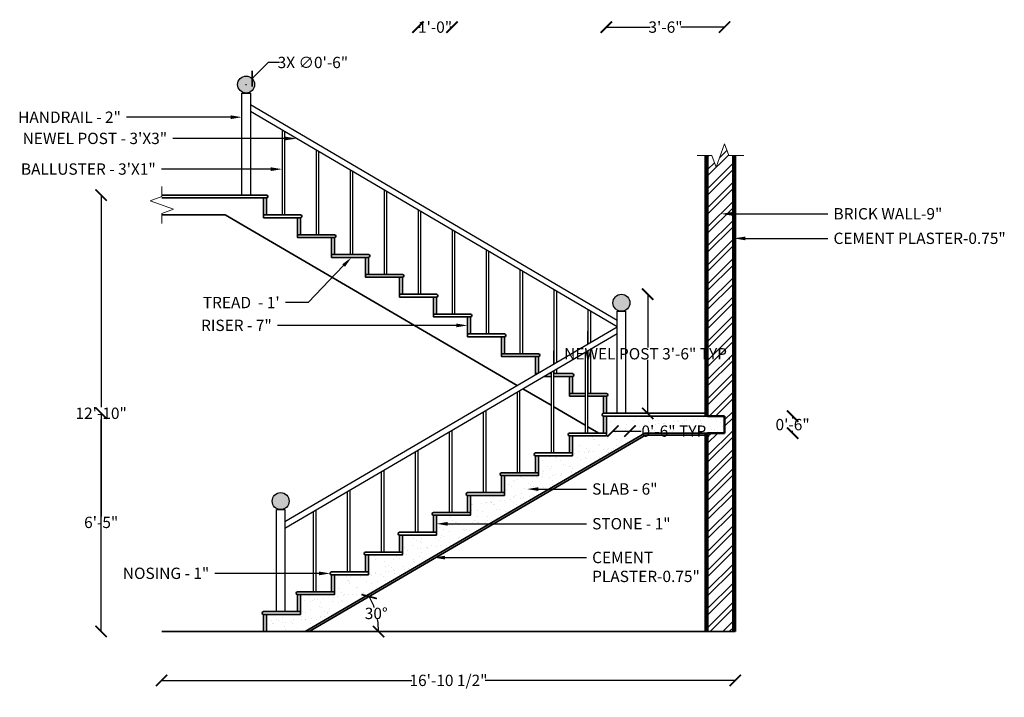
# Model space of a CAD drawing. Units: inches. Extents: x -27 to 693, y -28 to 216.
# Tile 2 of 2: x 345 to 693, y -23 to 216. Entities that reach past the tile are written whole.
import ezdxf
from ezdxf import colors
from ezdxf.entities.mleader import LeaderData, LeaderLine
from ezdxf.math import Vec2, Vec3

# ---------------------------------------------------------------- set-up
doc = ezdxf.new("R2010")
doc.units = ezdxf.units.IN
for name, color, linetype, lineweight in [('A-ANNO-DIMS', 2, 'Continuous', 18), ('A-ANNO-SYMB', 3, 'Continuous', 18), ('A-ANNO-TEXT', 7, 'Continuous', 18), ('A-FLOR-HRAL', 4, 'Continuous', 25), ('A-SECT', 7, 'Continuous', 35), ('A-SECT-PATT', 8, 'Continuous', 13), ('A-WALL', 7, 'Continuous', 50), ('A-WALL-PATT', 8, 'Continuous', 18)]:
    doc.layers.add(name, color=color, linetype=linetype, lineweight=lineweight)
doc.styles.get("Standard").update_dxf_attribs({"font": 'arial.ttf'})
doc.dimstyles.get("Standard").update_dxf_attribs({"dimtxt": 4, "dimasz": 4, "dimexe": 0.18, "dimexo": 0.0625, "dimgap": 0.09, "dimtad": 0, "dimtih": 1, "dimtoh": 1, "dimzin": 0, "dimdsep": 46, "dimlunit": 3, "dimtxsty": 'Standard', "dimblk": 'ARCHTICK', "dimcen": 0.09, "dimse1": 1, "dimse2": 1, "dimclrd": 4, "dimclrt": 2, "dimadec": 0, "dimazin": 0, "dimtfac": 1, "dimtofl": 0, "dimtmove": 0, "dimatfit": 3, "dimfxl": 1, "dimtolj": 1, "dimtzin": 0, "dimarcsym": 0})
pattern_1 = [(50, (395.0364, 293.9867), (1.821847, -0.159391), [0.1905, -2.0955]), (355, (395.0364, 293.9867), (-0.352434, 1.910568), [0.1524, -1.676406]), (100.45144, (395.1882, 293.9734), (1.4694125, 1.7511775), [0.1619, -1.780902]), (46.1842, (395.0364, 294.4947), (2.71079, -0.420423), [0.28575, -3.14325]), (96.6356, (395.2623, 294.4596), (2.374041, 2.474261), [0.24285, -2.671356]), (351.18415, (395.0364, 294.4947), (2.374041, 2.474261), [0.2286, -2.514597]), (21, (395.2904, 294.3677), (1.516144, -1.022652), [0.1905, -2.0955]), (326, (395.2904, 294.3677), (0.61802, 1.84188), [0.1524, -1.6764]), (71.45144, (395.4167, 294.2824), (2.134164, 0.819228), [0.1619, -1.780899]), (37.5, (395.03637, 293.98666), (0.030886, 0.8455504), [0, -1.65608, 0, -1.7018, 0, -1.68275]), (7.5, (395.0364, 293.9867), (0.6681966, 1.0018057), [0, -0.97028, 0, -1.61798, 0, -0.64135]), (327.5, (394.46995, 293.98666), (1.355906, -0.0572874), [0, -0.635, 0, -1.9812, 0, -2.6289]), (317.5, (394.216, 293.9867), (1.481292, 0.254265), [0, -0.8255, 0, -1.31572, 0, -1.8669])]

# ---------------------------------------------------------------- blocks, each defined once
blk = doc.blocks.new('_ArchTick')
at = {"color": 0, "linetype": 'ByBlock', "const_width": 0.15}
blk.add_lwpolyline([(-0.5, -0.5), (0.5, 0.5)], dxfattribs=at)
blk = doc.blocks.new('*D7')
at = {"layer": 'A-ANNO-DIMS', "color": 0, "lineweight": -2, "transparency": 16777216}
for start, end in [(20.3751, 30.2564), (0, 10.0085)]:
    blk.add_arc((447.16, 0.49), 24.47, start, end, dxfattribs=at)
at = {"layer": 'DEFPOINTS', "color": 0, "transparency": 16777216}
for p in [(565.88, 69.74), (471.26, 4.77), (395.05, 0.49), (447.16, 0.49), (597.55, 0.49)]:
    blk.add_point(p, dxfattribs=at)
at = {"layer": 'A-ANNO-DIMS', "color": 0, "lineweight": -2, "transparency": 16777216, "xscale": 4, "yscale": 4, "zscale": 4}
for p, rotation in [((468.3, 12.82), 120.2564371635292), ((471.64, 0.49), 270)]:
    blk.add_blockref('_ArchTick', p, dxfattribs=dict(at, rotation=rotation))
at = {"layer": 'A-ANNO-DIMS', "color": 0, "transparency": 16777216, "insert": (470.79, 6.87), "char_height": 4, "attachment_point": 5}
blk.add_mtext('\\A1;30°', dxfattribs=at)
blk = doc.blocks.new('NEWEL-POST')
h = blk.add_hatch(color=256)
h.dxf.hatch_style = 1
h.paths.add_polyline_path([(0, 39, 1), (6, 39, 1)])
blk.add_lwpolyline([(1.5, 36), (4.5, 36), (4.5, 0), (1.5, 0)], close=True)
blk.add_circle((3, 39), 3)
blk = doc.blocks.new('*D9')
at = {"layer": 'A-ANNO-DIMS', "color": 4, "lineweight": -2, "transparency": 16777216}
for p, q in [((566.65, 119.49), (566.65, 100.65)), ((566.65, 77.49), (566.65, 96.33))]:
    blk.add_line(p, q, dxfattribs=at)
at = {"layer": 'DEFPOINTS', "color": 0, "transparency": 16777216}
for p in [(560.35, 119.49), (566.65, 119.49), (560.35, 77.49)]:
    blk.add_point(p, dxfattribs=at)
at = {"layer": 'A-ANNO-DIMS', "color": 4, "lineweight": -2, "transparency": 16777216, "xscale": 4, "yscale": 4, "zscale": 4}
for p, rotation in [((566.65, 119.49), 90), ((566.65, 77.49), 270)]:
    blk.add_blockref('_ArchTick', p, dxfattribs=dict(at, rotation=rotation))
at = {"layer": 'A-ANNO-DIMS', "color": 2, "transparency": 16777216, "insert": (566.65, 98.49), "char_height": 4, "attachment_point": 5}
blk.add_mtext('\\A1;NEWEL POST 3\'-6" TYP.', dxfattribs=at)
blk = doc.blocks.new('*D10')
at = {"layer": 'A-ANNO-DIMS', "color": 4, "lineweight": -2, "transparency": 16777216}
for p, q in [((554.35, 71.19), (560.35, 71.19)), ((560.35, 71.19), (564.35, 71.19))]:
    blk.add_line(p, q, dxfattribs=at)
at = {"layer": 'DEFPOINTS', "color": 0, "transparency": 16777216}
for p in [(554.35, 77.49), (560.35, 77.49), (560.35, 71.19)]:
    blk.add_point(p, dxfattribs=at)
at = {"layer": 'A-ANNO-DIMS', "color": 4, "lineweight": -2, "transparency": 16777216, "xscale": 4, "yscale": 4, "zscale": 4, "rotation": 180}
blk.add_blockref('_ArchTick', (554.35, 71.19), dxfattribs=at)
at = {"layer": 'A-ANNO-DIMS', "color": 4, "lineweight": -2, "transparency": 16777216, "xscale": 4, "yscale": 4, "zscale": 4}
blk.add_blockref('_ArchTick', (560.35, 71.19), dxfattribs=at)
at = {"layer": 'A-ANNO-DIMS', "color": 2, "transparency": 16777216, "insert": (576.64, 71.19), "char_height": 4, "attachment_point": 5}
blk.add_mtext('\\A1;0\'-6" TYP.', dxfattribs=at)
blk = doc.blocks.new('*D16')
at = {"layer": 'A-ANNO-DIMS', "color": 4, "lineweight": -2, "transparency": 16777216}
for p, q in [((395.05, -16.76), (483.32, -16.76)), ((597.55, -16.76), (509.29, -16.76))]:
    blk.add_line(p, q, dxfattribs=at)
at = {"layer": 'DEFPOINTS', "color": 0, "transparency": 16777216}
for p in [(395.05, 0.49), (597.55, 0.49), (597.55, -16.76)]:
    blk.add_point(p, dxfattribs=at)
at = {"layer": 'A-ANNO-DIMS', "color": 4, "lineweight": -2, "transparency": 16777216, "xscale": 4, "yscale": 4, "zscale": 4, "rotation": 180}
blk.add_blockref('_ArchTick', (395.05, -16.76), dxfattribs=at)
at = {"layer": 'A-ANNO-DIMS', "color": 4, "lineweight": -2, "transparency": 16777216, "xscale": 4, "yscale": 4, "zscale": 4}
blk.add_blockref('_ArchTick', (597.55, -16.76), dxfattribs=at)
at = {"layer": 'A-ANNO-DIMS', "color": 2, "transparency": 16777216, "insert": (496.3, -16.76), "char_height": 4, "attachment_point": 5}
blk.add_mtext('\\A1;16\'-10 1/2"', dxfattribs=at)
blk = doc.blocks.new('*D17')
at = {"layer": 'A-ANNO-DIMS', "color": 4, "lineweight": -2, "transparency": 16777216}
for p, q in [((373.68, 154.49), (373.68, 79.62)), ((373.68, 0.49), (373.68, 75.35))]:
    blk.add_line(p, q, dxfattribs=at)
at = {"layer": 'DEFPOINTS', "color": 0, "transparency": 16777216}
for p in [(373.68, 154.49), (395.05, 154.49), (395.05, 0.49)]:
    blk.add_point(p, dxfattribs=at)
at = {"layer": 'A-ANNO-DIMS', "color": 4, "lineweight": -2, "transparency": 16777216, "xscale": 4, "yscale": 4, "zscale": 4}
for p, rotation in [((373.68, 154.49), 90), ((373.68, 0.49), 270)]:
    blk.add_blockref('_ArchTick', p, dxfattribs=dict(at, rotation=rotation))
at = {"layer": 'A-ANNO-DIMS', "color": 2, "transparency": 16777216, "insert": (373.68, 77.49), "char_height": 4, "attachment_point": 5}
blk.add_mtext('\\A1;12\'-10"', dxfattribs=at)
blk = doc.blocks.new('*D18')
at = {"layer": 'A-ANNO-DIMS', "color": 4, "lineweight": -2, "transparency": 16777216}
for p, q in [((373.68, 77.49), (373.68, 41.12)), ((373.68, 0.49), (373.68, 36.85))]:
    blk.add_line(p, q, dxfattribs=at)
at = {"layer": 'DEFPOINTS', "color": 0, "transparency": 16777216}
for p in [(373.68, 77.49), (552.05, 77.49), (395.05, 0.49)]:
    blk.add_point(p, dxfattribs=at)
at = {"layer": 'A-ANNO-DIMS', "color": 4, "lineweight": -2, "transparency": 16777216, "xscale": 4, "yscale": 4, "zscale": 4}
for p, rotation in [((373.68, 77.49), 90), ((373.68, 0.49), 270)]:
    blk.add_blockref('_ArchTick', p, dxfattribs=dict(at, rotation=rotation))
at = {"layer": 'A-ANNO-DIMS', "color": 2, "transparency": 16777216, "insert": (373.68, 38.99), "char_height": 4, "attachment_point": 5}
blk.add_mtext('\\A1;6\'-5"', dxfattribs=at)
blk = doc.blocks.new('*D19')
at = {"layer": 'A-ANNO-DIMS', "color": 4, "lineweight": -2, "transparency": 16777216}
for p, q in [((617.8, 76.49), (617.8, 75.62)), ((617.8, 70.49), (617.8, 71.35))]:
    blk.add_line(p, q, dxfattribs=at)
at = {"layer": 'DEFPOINTS', "color": 0, "transparency": 16777216}
for p in [(593.8, 76.49), (617.8, 76.49), (593.8, 70.49)]:
    blk.add_point(p, dxfattribs=at)
at = {"layer": 'A-ANNO-DIMS', "color": 4, "lineweight": -2, "transparency": 16777216, "xscale": 4, "yscale": 4, "zscale": 4}
for p, rotation in [((617.8, 76.49), 90), ((617.8, 70.49), 270)]:
    blk.add_blockref('_ArchTick', p, dxfattribs=dict(at, rotation=rotation))
at = {"layer": 'A-ANNO-DIMS', "color": 2, "transparency": 16777216, "insert": (617.8, 73.49), "char_height": 4, "attachment_point": 5}
blk.add_mtext('\\A1;0\'-6"', dxfattribs=at)
blk = doc.blocks.new('*D20')
at = {"layer": 'A-ANNO-DIMS', "color": 4, "lineweight": -2, "transparency": 16777216}
for p, q in [((552.05, 213.74), (567.52, 213.74)), ((593.8, 213.74), (578.33, 213.74))]:
    blk.add_line(p, q, dxfattribs=at)
at = {"layer": 'DEFPOINTS', "color": 0, "transparency": 16777216}
for p in [(593.8, 213.74), (552.05, 70.49), (593.8, 70.49)]:
    blk.add_point(p, dxfattribs=at)
at = {"layer": 'A-ANNO-DIMS', "color": 4, "lineweight": -2, "transparency": 16777216, "xscale": 4, "yscale": 4, "zscale": 4, "rotation": 180}
blk.add_blockref('_ArchTick', (552.05, 213.74), dxfattribs=at)
at = {"layer": 'A-ANNO-DIMS', "color": 4, "lineweight": -2, "transparency": 16777216, "xscale": 4, "yscale": 4, "zscale": 4}
blk.add_blockref('_ArchTick', (593.8, 213.74), dxfattribs=at)
at = {"layer": 'A-ANNO-DIMS', "color": 2, "transparency": 16777216, "insert": (572.93, 213.74), "char_height": 4, "attachment_point": 5}
blk.add_mtext('\\A1;3\'-6"', dxfattribs=at)
blk = doc.blocks.new('*D21')
at = {"layer": 'A-ANNO-DIMS', "color": 4, "lineweight": -2, "transparency": 16777216}
for p, q in [((485.55, 213.74), (486.33, 213.74)), ((497.55, 213.74), (496.77, 213.74))]:
    blk.add_line(p, q, dxfattribs=at)
at = {"layer": 'DEFPOINTS', "color": 0, "transparency": 16777216}
for p in [(497.55, 213.74), (485.55, 149.25), (497.55, 142.2)]:
    blk.add_point(p, dxfattribs=at)
at = {"layer": 'A-ANNO-DIMS', "color": 4, "lineweight": -2, "transparency": 16777216, "xscale": 4, "yscale": 4, "zscale": 4, "rotation": 180}
blk.add_blockref('_ArchTick', (485.55, 213.74), dxfattribs=at)
at = {"layer": 'A-ANNO-DIMS', "color": 4, "lineweight": -2, "transparency": 16777216, "xscale": 4, "yscale": 4, "zscale": 4}
blk.add_blockref('_ArchTick', (497.55, 213.74), dxfattribs=at)
at = {"layer": 'A-ANNO-DIMS', "color": 2, "transparency": 16777216, "insert": (491.55, 213.74), "char_height": 4, "attachment_point": 5}
blk.add_mtext('\\A1;1\'-0"', dxfattribs=at)
blk = doc.blocks.new('*D22')
at = {"layer": 'A-ANNO-DIMS', "color": 4, "lineweight": -2, "transparency": 16777216}
for p, q in [((432.65, 201.27), (426.99, 195.61)), ((436.65, 201.27), (432.65, 201.27))]:
    blk.add_line(p, q, dxfattribs=at)
at = {"layer": 'A-ANNO-DIMS', "color": 0, "lineweight": -2, "transparency": 16777216}
for p, q in [((424.78, 193.49), (424.96, 193.49)), ((424.87, 193.4), (424.87, 193.58))]:
    blk.add_line(p, q, dxfattribs=at)
at = {"layer": 'DEFPOINTS', "color": 0, "transparency": 16777216}
for p in [(426.99, 195.61), (422.75, 191.37)]:
    blk.add_point(p, dxfattribs=at)
at = {"layer": 'A-ANNO-DIMS', "color": 4, "lineweight": -2, "transparency": 16777216, "xscale": 4, "yscale": 4, "zscale": 4, "rotation": 224.998176859595}
blk.add_blockref('_ArchTick', (426.99, 195.61), dxfattribs=at)
at = {"layer": 'A-ANNO-DIMS', "color": 2, "transparency": 16777216, "insert": (448.42, 201.27), "char_height": 4, "attachment_point": 5}
blk.add_mtext('\\A1;3X ∅0\'-6"', dxfattribs=at)

msp = doc.modelspace()

# ---------------------------------------------------------------- hatches: boundary and pattern name
at = {"layer": 'A-SECT-PATT'}
h = msp.add_hatch(dxfattribs=at)
h.set_pattern_fill('AR-SAND', color=256, scale=0.1)
h.set_pattern_definition([(37.5, (395.0364, 293.9867), (-0.160003, 4.894132), [0, -3.8608, 0, -4.318, 0, -4.1275]), (7.5, (395.0364, 293.9867), (4.49523, 7.16825), [0, -2.0828, 0, -3.4798, 0, -1.3335]), (327.5, (391.912, 293.9867), (7.909924, 0.01437), [0, -1.27, 0, -4.572, 0, -5.969]), (317.5, (391.912, 293.9867), (7.63556, 2.22929), [0, -0.635, 0, -2.9972, 0, -3.429])])
h.paths.add_polyline_path([(516.053, 55.487), (516.053, 49.487), (516.053, 48.487), (515.053, 48.487), (504.053, 48.487), (504.053, 42.487), (504.053, 41.487), (503.053, 41.487), (492.053, 41.487), (492.053, 35.487), (492.053, 34.487), (491.053, 34.487), (480.053, 34.487), (480.053, 28.487), (480.053, 27.487), (479.053, 27.487), (468.053, 27.487), (468.053, 21.487), (468.053, 20.487), (467.053, 20.487), (456.053, 20.487), (456.053, 14.487), (456.053, 13.487), (455.053, 13.487), (444.053, 13.487), (444.053, 7.487), (444.053, 6.487), (443.053, 6.487), (432.053, 6.487), (432.053, 0.487), (445.675, 0.487), (565.675, 70.487), (587.803, 70.487), (593.803, 70.487), (593.803, 76.487), (587.803, 76.487), (552.053, 76.487), (552.053, 70.487), (552.053, 69.487), (551.053, 69.487), (540.053, 69.487), (540.053, 63.487), (540.053, 62.487), (539.053, 62.487), (528.053, 62.487), (528.053, 56.487), (528.053, 55.487), (527.053, 55.487)])
h = msp.add_hatch(dxfattribs=at)
h.set_pattern_fill('AR-CONC', color=256, scale=0.01)
h.set_pattern_definition(pattern_1)
h.paths.add_polyline_path([(445.675, 0.487), (447.164, 0.487), (565.878, 69.737), (587.053, 69.737), (587.053, 70.487), (565.675, 70.487)])
at = {"layer": 'A-WALL-PATT'}
h = msp.add_hatch(dxfattribs=at)
h.set_pattern_fill('ANSI32', color=256, scale=0.5)
h.set_pattern_definition([(45, (395.0364, 293.9867), (-3.367596, 3.367596), []), (45, (397.2814, 293.9867), (-3.367596, 3.367596), [])])
h.paths.add_polyline_path([(596.803, 168.487), (595.303, 168.487), (593.803, 172.608), (590.803, 164.366), (589.303, 168.487), (587.803, 168.487), (587.803, 76.487), (593.803, 76.487), (593.803, 70.487), (587.803, 70.487), (587.803, 0.487), (596.803, 0.487)])
h = msp.add_hatch(dxfattribs=at)
h.set_pattern_fill('AR-CONC', color=256, scale=0.01)
h.set_pattern_definition(pattern_1)
h.paths.add_polyline_path([(587.803, 70.487), (587.053, 70.487), (587.053, 0.487), (587.803, 0.487)])
h.paths.add_polyline_path([(587.803, 168.487), (587.053, 168.487), (587.053, 76.487), (587.803, 76.487)])
h.paths.add_polyline_path([(597.553, 168.487), (596.803, 168.487), (596.803, 0.487), (597.553, 0.487)])

# ---------------------------------------------------------------- linework, layer by layer
at = {"layer": 'A-ANNO-SYMB'}
for points in [[(584.053, 168.487), (589.303, 168.487), (590.803, 164.366), (593.803, 172.608), (595.303, 168.487), (600.553, 168.487)], [(395.053, 157.487), (395.053, 153.987), (390.932, 152.487), (399.174, 149.487), (395.053, 147.987), (395.053, 144.487)]]:
    msp.add_lwpolyline(points, dxfattribs=at)
at = {"layer": 'A-FLOR-HRAL'}
for points in [[(555.855, 110.262), (426.369, 186.346)], [(438.553, 39.276), (555.855, 107.942), (426.369, 184.026)], [(437.553, 177.455), (437.553, 147.487), (438.553, 147.487), (438.553, 176.867)], [(449.553, 170.404), (449.553, 140.487), (450.553, 140.487), (450.553, 169.816)], [(461.553, 163.353), (461.553, 133.487), (462.553, 133.487), (462.553, 162.765)], [(473.553, 156.302), (473.553, 126.487), (474.553, 126.487), (474.553, 155.714)], [(485.553, 149.251), (485.553, 119.487), (486.553, 119.487), (486.553, 148.663)], [(497.553, 142.199), (497.553, 112.487), (498.553, 112.487), (498.553, 141.612)], [(509.553, 135.148), (509.553, 105.487), (510.553, 105.487), (510.553, 134.561)], [(521.553, 128.097), (521.553, 98.487), (522.553, 98.487), (522.553, 127.51)], [(533.553, 121.046), (533.553, 94.887)], [(534.553, 95.472), (534.553, 120.459)], [(545.553, 113.995), (545.553, 101.912)], [(546.553, 102.497), (546.553, 113.408)], [(438.553, 36.958), (555.855, 105.625)], [(545.553, 101.912), (545.553, 106.487)], [(533.553, 94.887), (533.553, 99.487)], [(544.553, 99.009), (544.553, 70.487), (545.553, 70.487), (545.553, 99.594)], [(545.553, 99.594), (545.553, 84.487), (546.553, 84.487), (546.553, 100.179)], [(532.553, 91.984), (532.553, 63.487), (533.553, 63.487), (533.553, 92.569)], [(533.553, 92.569), (533.553, 91.487), (534.553, 91.487), (534.553, 93.155)], [(520.553, 87.333), (520.553, 87.277)], [(520.553, 84.959), (520.553, 56.487), (521.553, 56.487), (521.553, 85.545)], [(508.553, 77.935), (508.553, 49.487), (509.553, 49.487), (509.553, 78.52)], [(496.553, 70.91), (496.553, 42.487), (497.553, 42.487), (497.553, 71.496)], [(484.553, 63.886), (484.553, 35.487), (485.553, 35.487), (485.553, 64.471)], [(472.553, 56.861), (472.553, 28.487), (473.553, 28.487), (473.553, 57.446)], [(460.553, 49.836), (460.553, 21.487), (461.553, 21.487), (461.553, 50.422)], [(448.553, 42.812), (448.553, 14.487), (449.553, 14.487), (449.553, 43.397)]]:
    msp.add_lwpolyline(points, dxfattribs=at)
at = {"layer": 'A-SECT'}
for p, q in [((432.053, 154.487), (395.053, 154.487)), ((395.303, 153.487), (395.053, 153.487)), ((432.053, 153.487), (395.303, 153.487)), ((431.053, 147.487), (431.053, 153.487)), ((432.053, 147.487), (432.053, 153.487)), ((395.053, 147.487), (395.303, 147.487)), ((417.431, 147.487), (395.303, 147.487)), ((520.601, 87.305), (417.431, 147.487)), ((432.053, 147.487), (431.053, 147.487)), ((432.053, 147.487), (431.053, 147.487)), ((444.053, 147.487), (432.053, 147.487)), ((444.053, 146.487), (432.053, 146.487)), ((443.053, 140.487), (443.053, 146.487)), ((444.053, 140.487), (444.053, 146.487)), ((444.053, 140.487), (443.053, 140.487)), ((456.053, 140.487), (444.053, 140.487)), ((456.053, 139.487), (444.053, 139.487)), ((455.053, 133.487), (455.053, 139.487)), ((456.053, 133.487), (456.053, 139.487)), ((456.053, 133.487), (455.053, 133.487)), ((468.053, 133.487), (456.053, 133.487)), ((468.053, 132.487), (456.053, 132.487)), ((467.053, 126.487), (467.053, 132.487)), ((468.053, 126.487), (468.053, 132.487)), ((468.053, 126.487), (467.053, 126.487)), ((480.053, 126.487), (468.053, 126.487)), ((480.053, 125.487), (468.053, 125.487)), ((479.053, 119.487), (479.053, 125.487)), ((480.053, 119.487), (480.053, 125.487)), ((480.053, 119.487), (479.053, 119.487)), ((492.053, 119.487), (480.053, 119.487)), ((492.053, 118.487), (480.053, 118.487)), ((491.053, 112.487), (491.053, 118.487)), ((492.053, 112.487), (492.053, 118.487)), ((492.053, 112.487), (491.053, 112.487)), ((504.053, 112.487), (492.053, 112.487)), ((504.053, 111.487), (492.053, 111.487)), ((503.053, 105.487), (503.053, 111.487)), ((504.053, 105.487), (504.053, 111.487)), ((504.053, 105.487), (503.053, 105.487)), ((516.053, 105.487), (504.053, 105.487)), ((516.053, 104.487), (504.053, 104.487)), ((515.053, 98.487), (515.053, 104.487)), ((516.053, 98.487), (516.053, 104.487)), ((516.053, 98.487), (515.053, 98.487)), ((528.053, 98.487), (516.053, 98.487)), ((528.053, 97.487), (516.053, 97.487)), ((527.053, 91.487), (527.053, 97.487)), ((528.053, 91.667), (528.053, 97.487)), ((527.745, 91.487), (527.053, 91.487)), ((532.553, 90.487), (529.996, 90.487)), ((532.553, 91.487), (531.704, 91.487)), ((540.053, 91.487), (533.553, 91.487)), ((540.053, 90.487), (533.553, 90.487)), ((539.053, 84.487), (539.053, 90.487)), ((540.053, 84.487), (540.053, 90.487)), ((532.553, 80.333), (522.584, 86.148)), ((539.053, 83.487), (539.053, 84.487)), ((540.053, 84.487), (539.053, 84.487)), ((540.053, 83.487), (539.053, 83.487)), ((544.553, 84.487), (540.053, 84.487)), ((544.553, 83.487), (540.053, 83.487)), ((552.053, 84.487), (545.553, 84.487)), ((552.053, 83.487), (545.553, 83.487)), ((551.053, 77.487), (551.053, 83.487)), ((552.053, 77.487), (552.053, 83.487)), ((544.553, 73.333), (533.553, 79.749)), ((551.053, 77.487), (587.053, 77.487)), ((552.053, 77.487), (551.053, 77.487)), ((551.053, 70.487), (551.053, 76.487)), ((551.053, 76.487), (587.803, 76.487)), ((552.053, 70.487), (552.053, 76.487)), ((539.053, 70.487), (551.053, 70.487)), ((549.431, 70.487), (545.553, 72.749)), ((551.053, 70.487), (552.053, 70.487)), ((551.053, 70.487), (552.053, 70.487)), ((539.053, 63.487), (539.053, 69.487)), ((539.053, 69.487), (551.053, 69.487)), ((540.053, 63.487), (540.053, 69.487)), ((527.053, 63.487), (539.053, 63.487)), ((539.053, 63.487), (540.053, 63.487)), ((527.053, 56.487), (527.053, 62.487)), ((527.053, 62.487), (539.053, 62.487)), ((528.053, 56.487), (528.053, 62.487)), ((515.053, 56.487), (527.053, 56.487)), ((527.053, 56.487), (528.053, 56.487)), ((515.053, 49.487), (515.053, 55.487)), ((515.053, 55.487), (527.053, 55.487)), ((516.053, 49.487), (516.053, 55.487)), ((503.053, 49.487), (515.053, 49.487)), ((515.053, 49.487), (516.053, 49.487)), ((503.053, 42.487), (503.053, 48.487)), ((503.053, 48.487), (515.053, 48.487)), ((504.053, 42.487), (504.053, 48.487)), ((491.053, 42.487), (503.053, 42.487)), ((503.053, 42.487), (504.053, 42.487)), ((491.053, 35.487), (491.053, 41.487)), ((491.053, 41.487), (503.053, 41.487)), ((492.053, 35.487), (492.053, 41.487)), ((479.053, 35.487), (491.053, 35.487)), ((491.053, 35.487), (492.053, 35.487)), ((479.053, 28.487), (479.053, 34.487)), ((479.053, 34.487), (491.053, 34.487)), ((480.053, 28.487), (480.053, 34.487)), ((467.053, 28.487), (479.053, 28.487)), ((479.053, 28.487), (480.053, 28.487)), ((467.053, 21.487), (467.053, 27.487)), ((467.053, 27.487), (479.053, 27.487)), ((468.053, 21.487), (468.053, 27.487)), ((455.053, 21.487), (467.053, 21.487)), ((467.053, 21.487), (468.053, 21.487)), ((455.053, 14.487), (455.053, 20.487)), ((455.053, 20.487), (467.053, 20.487)), ((456.053, 14.487), (456.053, 20.487)), ((443.053, 14.487), (455.053, 14.487)), ((455.053, 14.487), (456.053, 14.487)), ((443.053, 7.487), (443.053, 13.487)), ((443.053, 13.487), (455.053, 13.487)), ((444.053, 7.487), (444.053, 13.487)), ((431.053, 7.487), (443.053, 7.487)), ((443.053, 7.487), (444.053, 7.487)), ((444.053, 6.487), (444.053, 7.487)), ((431.053, 0.487), (431.053, 6.487)), ((431.053, 6.487), (443.053, 6.487)), ((432.053, 0.487), (432.053, 6.487)), ((443.053, 6.487), (444.053, 6.487)), ((395.053, 0.487), (597.553, 0.487)), ((431.053, 0.487), (432.053, 0.487))]:
    msp.add_line(p, q, dxfattribs=at)
for points in [[(432.053, 146.487), (431.053, 146.487), (431.053, 147.487)], [(444.053, 139.487), (443.053, 139.487), (443.053, 140.487)], [(456.053, 132.487), (455.053, 132.487), (455.053, 133.487)], [(468.053, 125.487), (467.053, 125.487), (467.053, 126.487)], [(480.053, 118.487), (479.053, 118.487), (479.053, 119.487)], [(492.053, 111.487), (491.053, 111.487), (491.053, 112.487)], [(504.053, 104.487), (503.053, 104.487), (503.053, 105.487)], [(516.053, 97.487), (515.053, 97.487), (515.053, 98.487)], [(527.053, 91.082), (527.053, 91.487)], [(445.675, 0.487), (565.675, 70.487), (587.803, 70.487)], [(447.164, 0.487), (565.878, 69.737), (587.053, 69.737)], [(551.053, 69.487), (552.053, 69.487), (552.053, 70.487)], [(539.053, 62.487), (540.053, 62.487), (540.053, 63.487)], [(527.053, 55.487), (528.053, 55.487), (528.053, 56.487)], [(515.053, 48.487), (516.053, 48.487), (516.053, 49.487)], [(503.053, 41.487), (504.053, 41.487), (504.053, 42.487)], [(491.053, 34.487), (492.053, 34.487), (492.053, 35.487)], [(479.053, 27.487), (480.053, 27.487), (480.053, 28.487)], [(467.053, 20.487), (468.053, 20.487), (468.053, 21.487)], [(455.053, 13.487), (456.053, 13.487), (456.053, 14.487)]]:
    msp.add_lwpolyline(points, dxfattribs=at)
for centre, start, end in [((432.053, 153.987), 270, 90), ((444.053, 146.987), 270, 90), ((456.053, 139.987), 270, 90), ((468.053, 132.987), 270, 90), ((480.053, 125.987), 270, 90), ((492.053, 118.987), 270, 90), ((504.053, 111.987), 270, 90), ((516.053, 104.987), 270, 90), ((528.053, 97.987), 270, 90), ((540.053, 90.987), 270, 90), ((552.053, 83.987), 270, 90), ((551.053, 76.987), 90, 270), ((539.053, 69.987), 90, 270), ((527.053, 62.987), 90, 270), ((515.053, 55.987), 90, 270), ((503.053, 48.987), 90, 270), ((491.053, 41.987), 90, 270), ((479.053, 34.987), 90, 270), ((467.053, 27.987), 90, 270), ((455.053, 20.987), 90, 270), ((443.053, 13.987), 90, 270), ((431.053, 6.987), 90, 270)]:
    msp.add_arc(centre, 0.5, start, end, dxfattribs=at)
at = {"layer": 'A-WALL'}
for p, q in [((587.053, 76.487), (587.053, 168.487)), ((587.803, 76.487), (587.803, 168.487)), ((596.803, 0.487), (596.803, 168.487)), ((597.553, 0.487), (597.553, 168.487)), ((587.803, 76.487), (593.803, 76.487)), ((593.803, 76.487), (593.803, 70.487)), ((587.053, 70.487), (587.053, 0.487)), ((587.803, 70.487), (587.803, 0.487)), ((593.803, 70.487), (587.803, 70.487))]:
    msp.add_line(p, q, dxfattribs=at)

# ---------------------------------------------------------------- block references
at = {"layer": 'A-FLOR-HRAL'}
for p in [(421.869, 154.487), (554.355, 77.487), (434.053, 7.487)]:
    msp.add_blockref('NEWEL-POST', p, dxfattribs=at)

# ---------------------------------------------------------------- dimensions: what is measured, and where the dimension line sits
at = {"layer": 'A-ANNO-DIMS'}
for base, p1, p2, picture, middle in [((497.553, 213.737), (485.553, 149.251), (497.553, 142.199), '*D21', (491.553, 213.737)), ((593.803017, 213.737163), (552.053017, 70.487163), (593.803017, 70.487163), '*D20', (572.928017, 213.737163)), ((597.553, -16.763), (395.053, 0.487), (597.553, 0.487), '*D16', (496.303, -16.763))]:
    dim = msp.add_linear_dim(base=base, p1=p1, p2=p2, dimstyle='Standard', override={"dimdec": 1, "dimlfac": 1, "dimrnd": 0, "dimzin": 1, "dimdsep": 46, "dimlunit": 4, "dimfrac": 2}, dxfattribs=at)
    dim.commit()
    dim.dimension.update_dxf_attribs({"geometry": picture, "text_midpoint": middle})
dim = msp.add_diameter_dim_2p(p1=(422.748, 191.366), p2=(426.99, 195.608), text='3X <>', dimstyle='Standard', override={"dimdec": 1, "dimlfac": 1, "dimrnd": 0, "dimzin": 1, "dimdsep": 46, "dimlunit": 4, "dimfrac": 2}, dxfattribs=at)
dim.commit()
dim.dimension.update_dxf_attribs({"geometry": '*D22', "text_midpoint": (448.42, 201.265), "dimtype": 163})
for base, p1, p2, picture, middle in [((373.682, 154.487), (395.053, 0.487), (395.053, 154.487), '*D17', (373.682, 77.487)), ((373.682, 77.487), (395.053, 0.487), (552.053, 77.487), '*D18', (373.682, 38.987)), ((617.803, 76.487), (593.803, 70.487), (593.803, 76.487), '*D19', (617.803, 73.487))]:
    dim = msp.add_linear_dim(base=base, p1=p1, p2=p2, angle=90, dimstyle='Standard', override={"dimdec": 1, "dimlfac": 1, "dimrnd": 0, "dimzin": 1, "dimdsep": 46, "dimlunit": 4, "dimfrac": 2}, dxfattribs=at)
    dim.commit()
    dim.dimension.update_dxf_attribs({"geometry": picture, "text_midpoint": middle})
dim = msp.add_linear_dim(base=(566.655, 119.487), p1=(560.355, 77.487), p2=(560.355, 119.487), angle=90, text='NEWEL POST <> TYP.', dimstyle='Standard', override={"dimdec": 1, "dimrnd": 0, "dimzin": 1, "dimlunit": 4, "dimfrac": 2}, dxfattribs=at)
dim.commit()
dim.dimension.update_dxf_attribs({"geometry": '*D9', "text_midpoint": (566.655, 98.487)})
dim = msp.add_linear_dim(base=(560.355, 71.187), p1=(554.355, 77.487), p2=(560.355, 77.487), text='<> TYP.', dimstyle='Standard', override={"dimdec": 1, "dimrnd": 0, "dimzin": 1, "dimlunit": 4, "dimfrac": 2}, dxfattribs=at)
dim.commit()
dim.dimension.update_dxf_attribs({"geometry": '*D10', "text_midpoint": (576.636, 71.187)})
dim = msp.add_angular_dim_2l(base=(471.258, 4.773), line1=((395.053, 0.487), (597.553, 0.487)), line2=((447.164, 0.487), (565.878, 69.737)), dimstyle='Standard', override={"dimclrd": 0, "dimclre": 0, "dimclrt": 0}, dxfattribs=at)
dim.commit()
dim.dimension.update_dxf_attribs({"geometry": '*D7', "text_midpoint": (470.788, 6.874)})

# ---------------------------------------------------------------- leaders
at = {"layer": 'A-ANNO-TEXT'}
ml = msp.add_multileader_mtext('Standard', dxfattribs=at)
ml.set_content('HANDRAIL - 2"', color=256)
ml.set_leader_properties()
ml.build(insert=Vec2(0, 0))
ctx = ml.context
ctx.base_point, ctx.plane_origin = Vec3(341.049, 181.957), Vec3(423.369, 181.957)
ctx.text_align_type = 2
notes = []
notes.append((ctx, [(0, (1, 1, 0), (390.653, 181.957), (-1, 0), 8, [(0, [(423.369, 181.957)], 0, [])])]))
ctx.mtext.insert, ctx.mtext.alignment, ctx.mtext.flow_direction = Vec3(380.653, 183.958), 3, 5
ml = msp.add_multileader_mtext('Standard', dxfattribs=at)
ml.set_content('NEWEL POST - 3\'X3"', color=256)
ml.set_leader_properties()
ml.build(insert=Vec2(0, 0))
ctx = ml.context
ctx.base_point, ctx.plane_origin = Vec3(341.049, 174.445), Vec3(442.675, 174.445)
ctx.text_align_type = 2
notes.append((ctx, [(0, (1, 1, 0), (406.959, 174.445), (-1, 0), 8, [(0, [(442.675, 174.445)], 0, [])])]))
ctx.mtext.insert, ctx.mtext.alignment, ctx.mtext.flow_direction = Vec3(396.959, 176.481), 3, 5
ml = msp.add_multileader_mtext('Standard', dxfattribs=at)
ml.set_content('BALLUSTER - 3\'X1"', color=256)
ml.set_leader_properties()
ml.build(insert=Vec2(0, 0))
ctx = ml.context
ctx.base_point, ctx.plane_origin = Vec3(341.049, 163.631), Vec3(437.553, 163.631)
ctx.text_align_type = 2
notes.append((ctx, [(0, (1, 1, 0), (402.945, 163.631), (-1, 0), 8, [(0, [(437.553, 163.631)], 0, [])])]))
ctx.mtext.insert, ctx.mtext.alignment, ctx.mtext.flow_direction = Vec3(392.945, 165.666), 3, 5
ml = msp.add_multileader_mtext('Standard', dxfattribs=at)
ml.set_content('BRICK WALL-9"', color=256)
ml.set_leader_properties()
ml.build(insert=Vec2(0, 0))
ctx = ml.context
ctx.base_point, ctx.plane_origin = Vec3(630.245, 147.855), Vec3(592.56, 147.855)
notes.append((ctx, [(0, (1, 1, 0), (622.245, 147.855), (1, 0), 8, [(0, [(592.56, 147.855)], 0, [])])]))
ctx.mtext.insert, ctx.mtext.flow_direction = Vec3(632.245, 149.889), 5
ml = msp.add_multileader_mtext('Standard', dxfattribs=at)
ml.set_content('CEMENT PLASTER-0.75"', color=256)
ml.set_leader_properties()
ml.build(insert=Vec2(0, 0))
ctx = ml.context
ctx.base_point, ctx.plane_origin = Vec3(630.245, 139.191), Vec3(597.095, 139.191)
notes.append((ctx, [(0, (1, 1, 0), (622.245, 139.191), (1, 0), 8, [(0, [(597.095, 139.191)], 0, [])])]))
ctx.mtext.insert, ctx.mtext.flow_direction = Vec3(632.245, 141.225), 5
ml = msp.add_multileader_mtext('Standard', dxfattribs=at)
ml.set_content("TREAD  - 1'", color=256)
ml.set_leader_properties()
ml.build(insert=Vec2(0, 0))
ctx = ml.context
ctx.base_point, ctx.plane_origin = Vec3(405.47, 116.571), Vec3(462.053, 132.487)
ctx.text_align_type = 2
notes.append((ctx, [(1, (1, 1, 0), (446.708, 116.571), (-1, 0), 8, [(0, [(462.053, 132.487)], 0, [])])]))
ctx.mtext.insert, ctx.mtext.alignment, ctx.mtext.flow_direction = Vec3(436.708, 118.572), 3, 5
ml = msp.add_multileader_mtext('Standard', dxfattribs=at)
ml.set_content('RISER - 7"', color=256)
ml.set_leader_properties()
ml.build(insert=Vec2(0, 0))
ctx = ml.context
ctx.base_point, ctx.plane_origin = Vec3(405.47, 108.487), Vec3(503.053, 108.487)
ctx.text_align_type = 2
notes.append((ctx, [(0, (1, 1, 0), (443.903, 108.487), (-1, 0), 8, [(0, [(503.053, 108.487)], 0, [])])]))
ctx.mtext.insert, ctx.mtext.alignment, ctx.mtext.flow_direction = Vec3(433.903, 110.521), 3, 5
ml = msp.add_multileader_mtext('Standard', dxfattribs=at)
ml.set_content('SLAB - 6"', color=256)
ml.set_leader_properties()
ml.build(insert=Vec2(0, 0))
ctx = ml.context
ctx.base_point, ctx.plane_origin = Vec3(545.027, 50.741), Vec3(524.03, 50.741)
notes.append((ctx, [(0, (1, 1, 0), (537.027, 50.741), (1, 0), 8, [(0, [(524.03, 50.741)], 0, [])])]))
ctx.mtext.insert, ctx.mtext.flow_direction = Vec3(547.027, 52.775), 5
ml = msp.add_multileader_mtext('Standard', dxfattribs=at)
ml.set_content('STONE - 1"', color=256)
ml.set_leader_properties()
ml.build(insert=Vec2(0, 0))
ctx = ml.context
ctx.base_point, ctx.plane_origin = Vec3(545.027, 38.487), Vec3(492.053, 38.487)
notes.append((ctx, [(0, (1, 1, 0), (537.027, 38.487), (1, 0), 8, [(0, [(492.053, 38.487)], 0, [])])]))
ctx.mtext.insert, ctx.mtext.flow_direction = Vec3(547.027, 40.521), 5
ml = msp.add_multileader_mtext('Standard', dxfattribs=at)
ml.set_content('CEMENT \\PPLASTER-0.75"', color=256)
ml.set_leader_properties()
ml.build(insert=Vec2(0, 0))
ctx = ml.context
ctx.base_point, ctx.plane_origin = Vec3(545.027, 26.566), Vec3(491.117, 26.566)
notes.append((ctx, [(0, (1, 1, 0), (537.027, 26.566), (1, 0), 8, [(0, [(491.117, 26.566)], 0, [])])]))
ctx.mtext.insert, ctx.mtext.flow_direction = Vec3(547.027, 28.6), 5
ml = msp.add_multileader_mtext('Standard', dxfattribs=at)
ml.set_content('NOSING - 1"', color=256)
ml.set_leader_properties()
ml.build(insert=Vec2(0, 0))
ctx = ml.context
ctx.base_point, ctx.plane_origin = Vec3(378.424, 20.987), Vec3(454.553, 20.987)
ctx.text_align_type = 2
notes.append((ctx, [(0, (1, 1, 0), (421.837, 20.987), (-1, 0), 8, [(0, [(454.553, 20.987)], 0, [])])]))
ctx.mtext.insert, ctx.mtext.alignment, ctx.mtext.flow_direction = Vec3(411.837, 23.021), 3, 5
for ctx, leaders in notes:
    for number, flags, end, landing, length, lines in leaders:
        leader = LeaderData()
        leader.index, (leader.has_last_leader_line, leader.has_dogleg_vector, leader.attachment_direction) = number, flags
        leader.last_leader_point, leader.dogleg_vector, leader.dogleg_length = Vec3(end), Vec3(landing), length
        for number, points, colour, breaks in lines:
            line = LeaderLine()
            line.index, line.vertices, line.color, line.breaks = number, Vec3.list(points), colors.encode_raw_color(colour), breaks
            leader.lines.append(line)
        ctx.leaders.append(leader)

doc.saveas('drawing.dxf')
